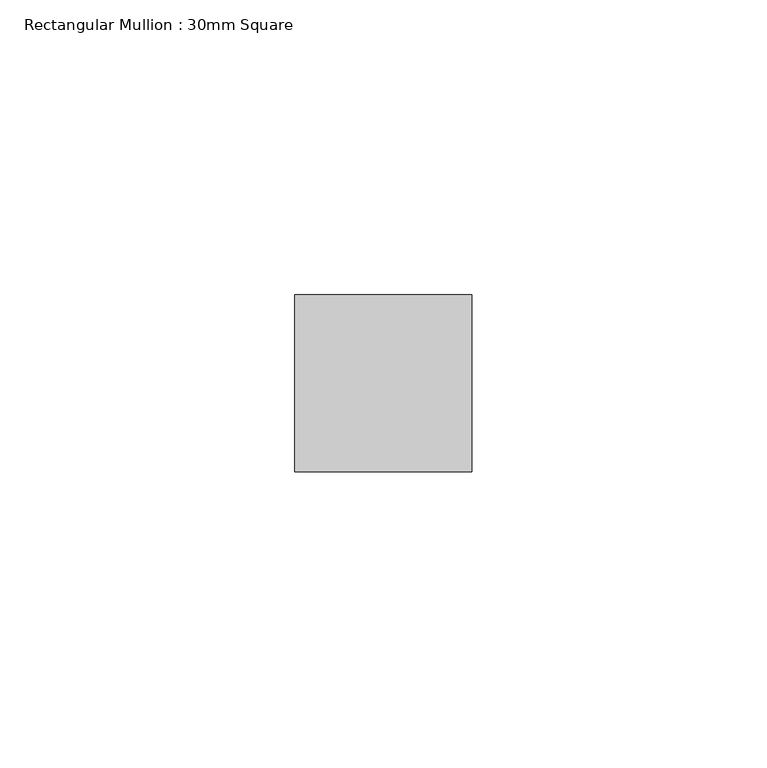
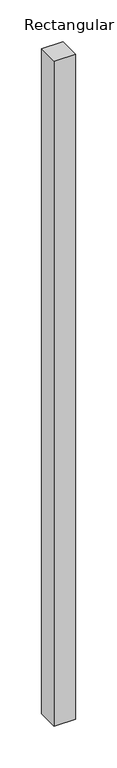
"""IFC4 building model written with IfcOpenShell, lengths in millimetres: member geometry, Rectangular Mullion : 30mm Square."""

from ifc_helpers import new_model, si_unit, frame, origin, place, context, project, spatial, polyline, outline, extrude, source, transform, mapped, element, save


def rectangular_mullion_30mm_square_2b64bb93(model_context):
    return source(origin(), model_context, "Body", "SweptSolid", [
        extrude(outline(polyline([(0.0, 15.0), (0.0, -15.0), (-30.0, -15.0), (-30.0, 15.0), (0.0, 15.0)])), frame((0.0, 0.0, -975.0), z_axis=(0.0, 0.0, 1.0), x_axis=(1.0, 0.0, 0.0)), (0.0, 0.0, 1.0), 975.0),
    ])


if __name__ == "__main__":
    model = new_model("IFC4")
    model_context = context("Model", 3, world=origin())
    ifc_project = project(units=[si_unit("LENGTHUNIT", "METRE", prefix="MILLI")], contexts=[model_context])
    site = spatial("IfcSite", under=ifc_project)
    building = spatial("IfcBuilding", under=site)
    placement = place(None, origin())
    rectangular_mullion_30mm_square_shape = rectangular_mullion_30mm_square_2b64bb93(model_context)
    element("IfcMember", 1, ObjectType="Rectangular Mullion : 30mm Square", at=placement, inside=building, context=model_context, shape_type="MappedRepresentation", body=[
        mapped(rectangular_mullion_30mm_square_shape, transform((0.0, 0.0, 0.0), x_axis=(1.0, 0.0, 0.0), y_axis=(0.0, 1.0, 0.0), z_axis=(0.0, 0.0, 1.0))),
    ])
    save(model, "model.ifc")

# Revit data of these elements
# Type "Rectangular Mullion : 30mm Square"
#   built-in parameter 1007304 = 0.0984252 (stored number, unit not read)
#   built-in parameter 1007301 = 0.0492126 (stored number, unit not read)
#   built-in parameter 1007300 = 0.0492126 (stored number, unit not read)
# Element 1 (IfcMember, "Rectangular Mullion : 30mm Square")
#   Materials on its faces: "Aluminum"
# Materials
#   "Aluminum": class "Metal", colour RGB 244 244 244, transparency 0, Description = "Aluminum 6061", Cost = 0
